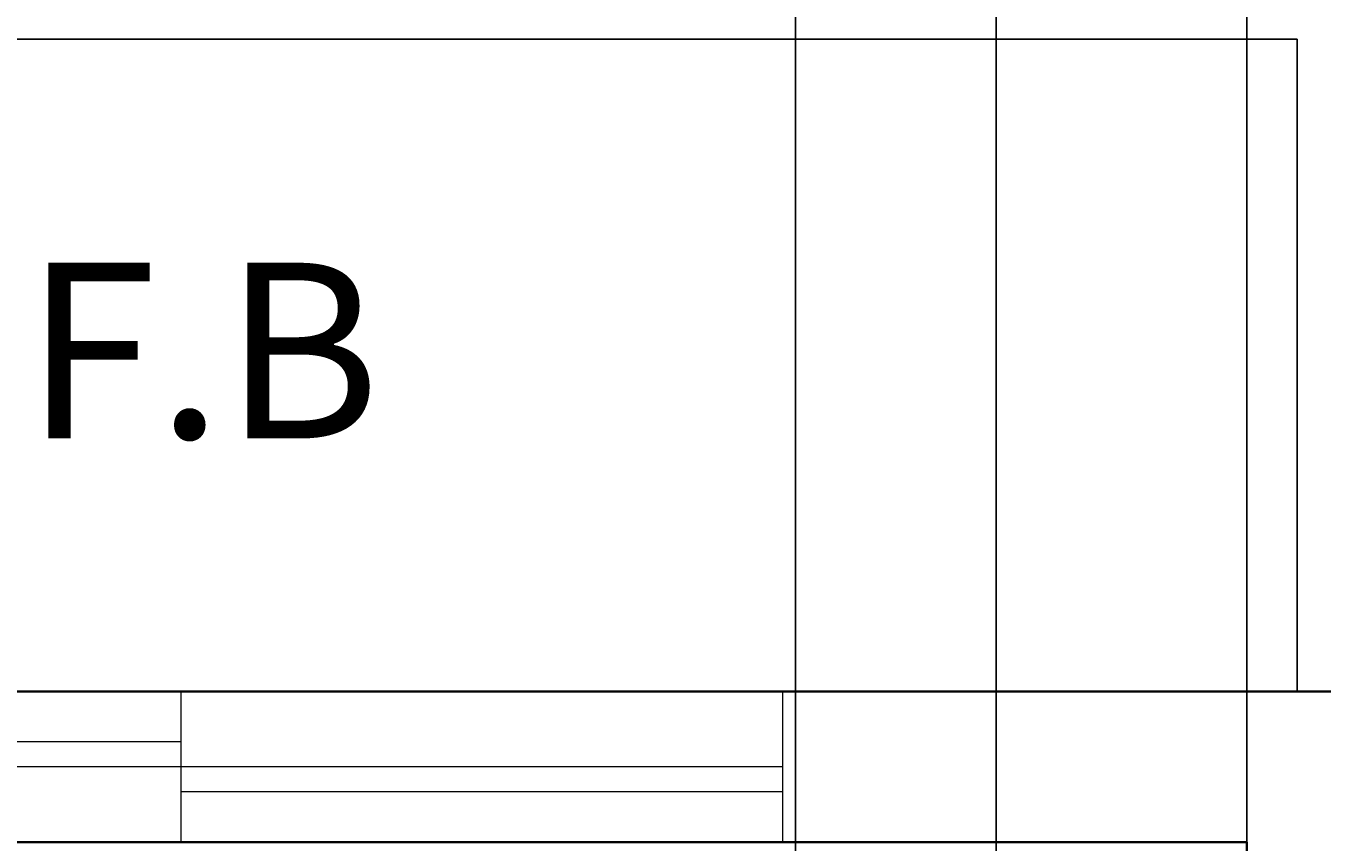
# Model space of a CAD drawing. Units: feet. Extents: x 105 to 1094, y -88 to 588.
# Tile 33 of 59: x 384 to 436, y 491 to 524. Entities that reach past the tile are written whole.
import ezdxf

# ---------------------------------------------------------------- set-up
doc = ezdxf.new("R2010")
doc.units = ezdxf.units.FT
doc.header["$MEASUREMENT"] = 0
for name, color, linetype, lineweight in [('A-ANNO-DIMS', 2, 'Continuous', 18), ('A-ANNO-TEXT', 7, 'Continuous', 18), ('A-FLOR-PROJ', 8, 'Continuous', 25), ('A-GLAZ', 4, 'Continuous', 18), ('A-WALL', 7, 'Continuous', 35)]:
    doc.layers.add(name, color=color, linetype=linetype, lineweight=lineweight)
doc.styles.get("Standard").update_dxf_attribs({"font": 'arial.ttf'})
doc.dimstyles.get("Standard").update_dxf_attribs({"dimtxt": 0.18, "dimasz": 0.18, "dimexe": 0.18, "dimexo": 0.0625, "dimgap": 0.09, "dimtad": 0, "dimtih": 1, "dimtoh": 1, "dimdec": 4, "dimzin": 0, "dimdsep": 46, "dimtxsty": 'Standard', "dimcen": 0.09, "dimadec": 0, "dimazin": 0, "dimtfac": 1, "dimtdec": 4, "dimtofl": 0, "dimtmove": 0, "dimatfit": 3, "dimfxl": 1, "dimtolj": 1, "dimtzin": 0, "dimarcsym": 0})

# ---------------------------------------------------------------- blocks, each defined once
blk = doc.blocks.new('WIN-TWO-LIGHT')
for p, q in [((0, 0), (0, 6)), ((24, 0), (24, 6)), ((48, 0), (48, 6)), ((24, 4), (48, 4)), ((0, 3), (48, 3)), ((0, 2), (24, 2))]:
    blk.add_line(p, q)
blk = doc.blocks.new('*D21')
at = {"layer": 'A-ANNO-DIMS', "color": 0, "lineweight": -2, "transparency": 16777216}
for p, q in [((849.626, 543.081), (105.458, 543.081)), ((105.638, 542.901), (105.638, 250.263)), ((105.638, -42.739), (105.638, 249.899)), ((849.626, -42.919), (105.458, -42.919))]:
    blk.add_line(p, q, dxfattribs=at)
at = {"layer": 'A-ANNO-DIMS', "color": 0, "transparency": 16777216}
for points in [[(105.608, 542.901), (105.668, 542.901), (105.638, 543.081)], [(105.608, -42.739), (105.668, -42.739), (105.638, -42.919)]]:
    blk.add_solid(points, dxfattribs=at)
at = {"layer": 'Defpoints', "color": 0, "transparency": 16777216}
for p in [(105.638, 543.081), (849.688, 543.081), (849.688, -42.919)]:
    blk.add_point(p, dxfattribs=at)
at = {"layer": 'A-ANNO-DIMS', "color": 0, "transparency": 16777216, "insert": (105.638, 250.081), "char_height": 0.18, "attachment_point": 5}
blk.add_mtext('\\A1;586', dxfattribs=at)
blk = doc.blocks.new('*D52')
at = {"layer": 'A-ANNO-DIMS', "color": 0, "lineweight": -2, "transparency": 16777216}
for p, q in [((414.688, 394.144), (414.688, 588.311)), ((432.688, 394.144), (432.688, 588.311)), ((414.868, 588.131), (423.478, 588.131)), ((432.508, 588.131), (423.899, 588.131))]:
    blk.add_line(p, q, dxfattribs=at)
at = {"layer": 'A-ANNO-DIMS', "color": 0, "transparency": 16777216}
for points in [[(414.868, 588.161), (414.868, 588.101), (414.688, 588.131)], [(432.508, 588.161), (432.508, 588.101), (432.688, 588.131)]]:
    blk.add_solid(points, dxfattribs=at)
at = {"layer": 'Defpoints', "color": 0, "transparency": 16777216}
for p in [(414.688, 588.131), (414.688, 394.081), (432.688, 394.081)]:
    blk.add_point(p, dxfattribs=at)
at = {"layer": 'A-ANNO-DIMS', "color": 0, "transparency": 16777216, "insert": (423.688, 588.131), "char_height": 0.18, "attachment_point": 5}
blk.add_mtext('\\A1;18', dxfattribs=at)
blk = doc.blocks.new('*D53')
at = {"layer": 'A-ANNO-DIMS', "color": 0, "lineweight": -2, "transparency": 16777216}
for p, q in [((365.688, 394.144), (365.688, 588.311)), ((414.688, 394.144), (414.688, 588.311)), ((365.868, 588.131), (389.966, 588.131)), ((414.508, 588.131), (390.411, 588.131))]:
    blk.add_line(p, q, dxfattribs=at)
at = {"layer": 'A-ANNO-DIMS', "color": 0, "transparency": 16777216}
for points in [[(365.868, 588.161), (365.868, 588.101), (365.688, 588.131)], [(414.508, 588.161), (414.508, 588.101), (414.688, 588.131)]]:
    blk.add_solid(points, dxfattribs=at)
at = {"layer": 'Defpoints', "color": 0, "transparency": 16777216}
for p in [(365.688, 588.131), (365.688, 394.081), (414.688, 394.081)]:
    blk.add_point(p, dxfattribs=at)
at = {"layer": 'A-ANNO-DIMS', "color": 0, "transparency": 16777216, "insert": (390.188, 588.131), "char_height": 0.18, "attachment_point": 5}
blk.add_mtext('\\A1;49', dxfattribs=at)
blk = doc.blocks.new('*D56')
at = {"layer": 'A-ANNO-DIMS', "color": 0, "lineweight": -2, "transparency": 16777216}
for p, q in [((374.688, 252.144), (374.688, 588.311)), ((422.688, 252.144), (422.688, 588.311)), ((374.868, 588.131), (398.466, 588.131)), ((422.508, 588.131), (398.911, 588.131))]:
    blk.add_line(p, q, dxfattribs=at)
at = {"layer": 'A-ANNO-DIMS', "color": 0, "transparency": 16777216}
for points in [[(374.868, 588.161), (374.868, 588.101), (374.688, 588.131)], [(422.508, 588.161), (422.508, 588.101), (422.688, 588.131)]]:
    blk.add_solid(points, dxfattribs=at)
at = {"layer": 'Defpoints', "color": 0, "transparency": 16777216}
for p in [(422.688, 588.131), (374.688, 252.081), (422.688, 252.081)]:
    blk.add_point(p, dxfattribs=at)
at = {"layer": 'A-ANNO-DIMS', "color": 0, "transparency": 16777216, "insert": (398.688, 588.131), "char_height": 0.18, "attachment_point": 5}
blk.add_mtext('\\A1;48', dxfattribs=at)

msp = doc.modelspace()

# ---------------------------------------------------------------- linework, layer by layer
at = {"layer": 'A-FLOR-PROJ'}
for q in [(349.6883, 523.0812), (434.6883, 497.0812)]:
    msp.add_line((434.6883, 523.0812), q, dxfattribs=at)
at = {"layer": 'A-WALL'}
for p, q in [((438.6883, 497.0812), (349.6883, 497.0812)), ((432.6883, 491.0812), (347.6883, 491.0812)), ((432.6883, 491.0812), (432.6883, 394.0812))]:
    msp.add_line(p, q, dxfattribs=at)

# ---------------------------------------------------------------- block references
at = {"layer": 'A-GLAZ', "extrusion": (0, 0, -1), "zscale": -1}
msp.add_blockref('WIN-TWO-LIGHT', (-414.1886, 491.081), dxfattribs=at)

# ---------------------------------------------------------------- texts
at = {"layer": 'A-ANNO-TEXT', "insert": (440.205, 514.1723), "char_height": 7, "attachment_point": 3}
msp.add_mtext_dynamic_manual_height_columns('\\pxqc;F.B ', width=98.34246, gutter_width=1, heights=[0], dxfattribs=at)

# ---------------------------------------------------------------- dimensions: what is measured, and where the dimension line sits
at = {"layer": 'A-ANNO-DIMS'}
for base, p1, p2, picture, middle in [((365.6883, 588.1312), (414.6883, 394.0812), (365.6883, 394.0812), '*D53', (390.1883, 588.1312)), ((422.6883, 588.1312), (374.6883, 252.0812), (422.6883, 252.0812), '*D56', (398.6883, 588.1312)), ((414.6883, 588.1312), (432.6883, 394.0812), (414.6883, 394.0812), '*D52', (423.6883, 588.1312))]:
    dim = msp.add_linear_dim(base=base, p1=p1, p2=p2, dimstyle='Standard', override={"dimdec": 0, "dimlfac": 1, "dimrnd": 0, "dimzin": 0, "dimdsep": 46, "dimlunit": 2}, dxfattribs=at)
    dim.commit()
    dim.dimension.update_dxf_attribs({"geometry": picture, "text_midpoint": middle})
dim = msp.add_linear_dim(base=(105.6383, 543.0812), p1=(849.6883, -42.9188), p2=(849.6883, 543.0812), angle=90, dimstyle='Standard', override={"dimdec": 0, "dimlfac": 1, "dimrnd": 0, "dimzin": 0, "dimdsep": 46, "dimlunit": 2}, dxfattribs=at)
dim.commit()
dim.dimension.update_dxf_attribs({"geometry": '*D21', "text_midpoint": (105.6383, 250.0812)})

doc.saveas('drawing.dxf')
